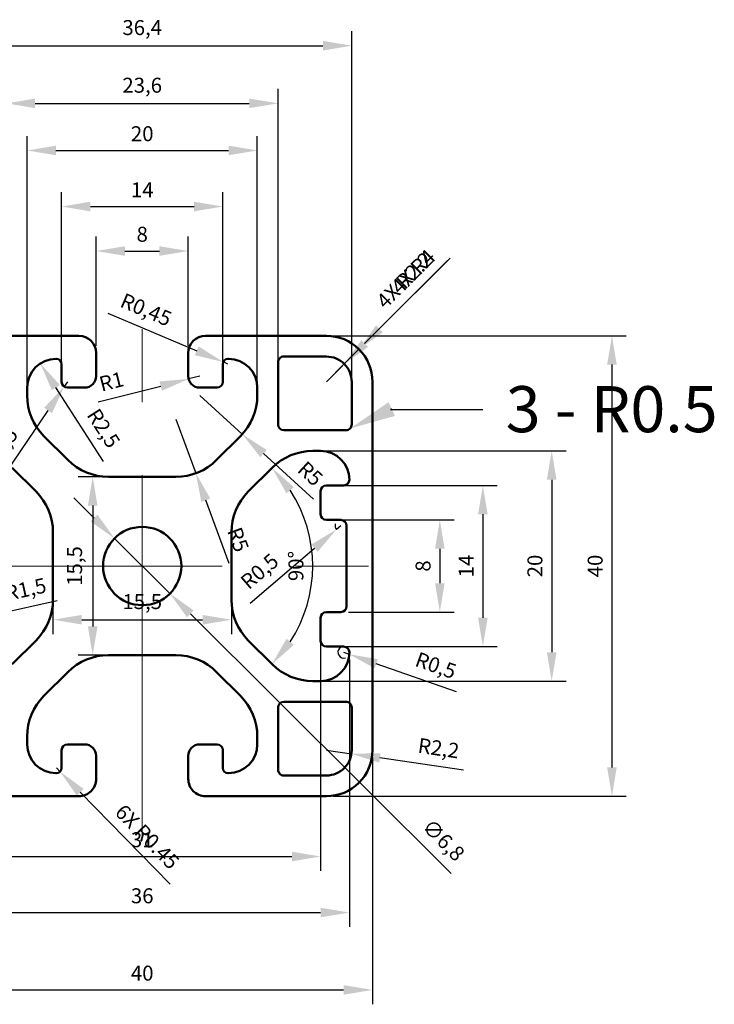
# Model space of a CAD drawing. Units: millimetres. Extents: x 2580.1 to 2672.5, y 2225.2 to 2310.7.
# Tile 2 of 2: x 2612.2 to 2672.5, y 2225.2 to 2310.7. Entities that reach past the tile are written whole.
import ezdxf
from ezdxf import colors
from ezdxf.entities.mleader import LeaderData, LeaderLine
from ezdxf.math import Vec2, Vec3

# ---------------------------------------------------------------- set-up
doc = ezdxf.new("R2010")
doc.units = ezdxf.units.MM
doc.linetypes.add('CENTER', pattern=[50.8, 31.75, -6.35, 6.35, -6.35])
for name, color, linetype, lineweight in [('M-CNTR', 1, 'CENTER', 18), ('M-DIMS', 2, 'Continuous', 25), ('M-OUTL', 7, 'Continuous', 50), ('M-TEXT', 3, 'Continuous', 25)]:
    doc.layers.add(name, color=color, linetype=linetype, lineweight=lineweight)
doc.styles.get("Standard").update_dxf_attribs({"font": 'arial.ttf'})
doc.dimstyles.new('ISO-25', dxfattribs={"dimtxt": 1.3, "dimasz": 2.5, "dimexe": 1.25, "dimexo": 0.625, "dimtad": 1, "dimtxsty": 'Standard', "dimcen": 2.5, "dimadec": 0, "dimazin": 0, "dimtfac": 1, "dimtmove": 0, "dimatfit": 3, "dimfxl": 1, "dimarcsym": 0})

# ---------------------------------------------------------------- blocks, each defined once
blk = doc.blocks.new('*D1')
at = {"layer": 'Defpoints', "color": 0, "transparency": 16777216}
for p in [(2626.849, 2290.611), (2618.849, 2281.743), (2626.849, 2281.743)]:
    blk.add_point(p, dxfattribs=at)
at = {"layer": 'M-DIMS', "color": 0, "lineweight": -2, "transparency": 16777216}
for p, q in [((2618.849, 2282.368), (2618.849, 2291.861)), ((2626.849, 2282.368), (2626.849, 2291.861)), ((2621.349, 2290.611), (2624.349, 2290.611))]:
    blk.add_line(p, q, dxfattribs=at)
at = {"layer": 'M-DIMS', "color": 0, "transparency": 16777216}
for points in [[(2621.349, 2291.028), (2621.349, 2290.194), (2618.849, 2290.611)], [(2624.349, 2291.028), (2624.349, 2290.194), (2626.849, 2290.611)]]:
    blk.add_solid(points, dxfattribs=at)
at = {"layer": 'M-DIMS', "color": 0, "transparency": 16777216, "insert": (2622.849, 2291.9), "char_height": 1.3, "attachment_point": 5}
blk.add_mtext('8', dxfattribs=at)
blk = doc.blocks.new('*D2')
at = {"layer": 'Defpoints', "color": 0, "transparency": 16777216}
for p in [(2629.849, 2294.477), (2615.849, 2280.018), (2629.849, 2280.018)]:
    blk.add_point(p, dxfattribs=at)
at = {"layer": 'M-DIMS', "color": 0, "lineweight": -2, "transparency": 16777216}
for p, q in [((2615.849, 2280.643), (2615.849, 2295.727)), ((2629.849, 2280.643), (2629.849, 2295.727)), ((2618.349, 2294.477), (2627.349, 2294.477))]:
    blk.add_line(p, q, dxfattribs=at)
at = {"layer": 'M-DIMS', "color": 0, "transparency": 16777216}
for points in [[(2618.349, 2294.894), (2618.349, 2294.061), (2615.849, 2294.477)], [(2627.349, 2294.894), (2627.349, 2294.061), (2629.849, 2294.477)]]:
    blk.add_solid(points, dxfattribs=at)
at = {"layer": 'M-DIMS', "color": 0, "transparency": 16777216, "insert": (2622.849, 2295.755), "char_height": 1.3, "attachment_point": 5}
blk.add_mtext('14', dxfattribs=at)
blk = doc.blocks.new('*D3')
at = {"layer": 'Defpoints', "color": 0, "transparency": 16777216}
for p in [(2632.849, 2299.349), (2612.849, 2278.404), (2632.849, 2278.404)]:
    blk.add_point(p, dxfattribs=at)
at = {"layer": 'M-DIMS', "color": 0, "lineweight": -2, "transparency": 16777216}
for p, q in [((2612.849, 2279.029), (2612.849, 2300.599)), ((2632.849, 2279.029), (2632.849, 2300.599)), ((2615.349, 2299.349), (2630.349, 2299.349))]:
    blk.add_line(p, q, dxfattribs=at)
at = {"layer": 'M-DIMS', "color": 0, "transparency": 16777216}
for points in [[(2615.349, 2299.766), (2615.349, 2298.932), (2612.849, 2299.349)], [(2630.349, 2299.766), (2630.349, 2298.932), (2632.849, 2299.349)]]:
    blk.add_solid(points, dxfattribs=at)
at = {"layer": 'M-DIMS', "color": 0, "transparency": 16777216, "insert": (2622.849, 2300.638), "char_height": 1.3, "attachment_point": 5}
blk.add_mtext('20', dxfattribs=at)
blk = doc.blocks.new('*D4')
at = {"layer": 'Defpoints', "color": 0, "transparency": 16777216}
for p in [(2634.649, 2303.442), (2611.049, 2278.243), (2634.649, 2278.243)]:
    blk.add_point(p, dxfattribs=at)
at = {"layer": 'M-DIMS', "color": 0, "lineweight": -2, "transparency": 16777216}
for p, q in [((2611.049, 2278.868), (2611.049, 2304.692)), ((2634.649, 2278.868), (2634.649, 2304.692)), ((2613.549, 2303.442), (2632.149, 2303.442))]:
    blk.add_line(p, q, dxfattribs=at)
at = {"layer": 'M-DIMS', "color": 0, "transparency": 16777216}
for points in [[(2613.549, 2303.859), (2613.549, 2303.026), (2611.049, 2303.442)], [(2632.149, 2303.859), (2632.149, 2303.026), (2634.649, 2303.442)]]:
    blk.add_solid(points, dxfattribs=at)
at = {"layer": 'M-DIMS', "color": 0, "transparency": 16777216, "insert": (2622.849, 2304.849), "char_height": 1.3, "attachment_point": 5}
blk.add_mtext('23,6', dxfattribs=at)
blk = doc.blocks.new('*D5')
at = {"layer": 'Defpoints', "color": 0, "transparency": 16777216}
for p in [(2641.049, 2308.452), (2604.649, 2277.393), (2641.049, 2277.393)]:
    blk.add_point(p, dxfattribs=at)
at = {"layer": 'M-DIMS', "color": 0, "lineweight": -2, "transparency": 16777216}
for p, q in [((2604.649, 2278.018), (2604.649, 2309.702)), ((2641.049, 2278.018), (2641.049, 2309.702)), ((2607.149, 2308.452), (2638.549, 2308.452))]:
    blk.add_line(p, q, dxfattribs=at)
at = {"layer": 'M-DIMS', "color": 0, "transparency": 16777216}
for points in [[(2607.149, 2308.869), (2607.149, 2308.036), (2604.649, 2308.452)], [(2638.549, 2308.869), (2638.549, 2308.036), (2641.049, 2308.452)]]:
    blk.add_solid(points, dxfattribs=at)
at = {"layer": 'M-DIMS', "color": 0, "transparency": 16777216, "insert": (2622.849, 2309.859), "char_height": 1.3, "attachment_point": 5}
blk.add_mtext('36,4', dxfattribs=at)
blk = doc.blocks.new('*D11')
at = {"layer": 'Defpoints', "color": 0, "transparency": 16777216}
for p in [(2602.849, 2247.243), (2642.849, 2247.243), (2642.849, 2226.409)]:
    blk.add_point(p, dxfattribs=at)
at = {"layer": 'M-DIMS', "color": 0, "lineweight": -2, "transparency": 16777216}
for p, q in [((2602.849, 2246.618), (2602.849, 2225.159)), ((2642.849, 2246.618), (2642.849, 2225.159)), ((2605.349, 2226.409), (2640.349, 2226.409))]:
    blk.add_line(p, q, dxfattribs=at)
at = {"layer": 'M-DIMS', "color": 0, "transparency": 16777216}
for points in [[(2605.349, 2226.826), (2605.349, 2225.992), (2602.849, 2226.409)], [(2640.349, 2226.826), (2640.349, 2225.992), (2642.849, 2226.409)]]:
    blk.add_solid(points, dxfattribs=at)
at = {"layer": 'M-DIMS', "color": 0, "transparency": 16777216, "insert": (2622.849, 2227.698), "char_height": 1.3, "attachment_point": 5}
blk.add_mtext('40', dxfattribs=at)
blk = doc.blocks.new('*D12')
at = {"layer": 'Defpoints', "color": 0, "transparency": 16777216}
for p in [(2607.349, 2257.493), (2638.349, 2257.493), (2638.349, 2238.001)]:
    blk.add_point(p, dxfattribs=at)
at = {"layer": 'M-DIMS', "color": 0, "lineweight": -2, "transparency": 16777216}
for p, q in [((2607.349, 2256.868), (2607.349, 2236.751)), ((2638.349, 2256.868), (2638.349, 2236.751)), ((2609.849, 2238.001), (2635.849, 2238.001))]:
    blk.add_line(p, q, dxfattribs=at)
at = {"layer": 'M-DIMS', "color": 0, "transparency": 16777216}
for points in [[(2609.849, 2238.418), (2609.849, 2237.584), (2607.349, 2238.001)], [(2635.849, 2238.418), (2635.849, 2237.584), (2638.349, 2238.001)]]:
    blk.add_solid(points, dxfattribs=at)
at = {"layer": 'M-DIMS', "color": 0, "transparency": 16777216, "insert": (2622.849, 2239.29), "char_height": 1.3, "attachment_point": 5}
blk.add_mtext('31', dxfattribs=at)
blk = doc.blocks.new('*D13')
at = {"layer": 'Defpoints', "color": 0, "transparency": 16777216}
for p in [(2604.85, 2255.804), (2640.849, 2255.743), (2640.849, 2233.131)]:
    blk.add_point(p, dxfattribs=at)
at = {"layer": 'M-DIMS', "color": 0, "lineweight": -2, "transparency": 16777216}
for p, q in [((2604.85, 2255.179), (2604.85, 2231.881)), ((2640.849, 2255.118), (2640.849, 2231.881)), ((2607.35, 2233.131), (2638.349, 2233.131))]:
    blk.add_line(p, q, dxfattribs=at)
at = {"layer": 'M-DIMS', "color": 0, "transparency": 16777216}
for points in [[(2607.35, 2233.547), (2607.35, 2232.714), (2604.85, 2233.131)], [(2638.349, 2233.547), (2638.349, 2232.714), (2640.849, 2233.131)]]:
    blk.add_solid(points, dxfattribs=at)
at = {"layer": 'M-DIMS', "color": 0, "transparency": 16777216, "insert": (2622.85, 2234.42), "char_height": 1.3, "attachment_point": 5}
blk.add_mtext('36', dxfattribs=at)
blk = doc.blocks.new('*D14')
at = {"layer": 'Defpoints', "color": 0, "transparency": 16777216}
for p in [(2639.474, 2267.243), (2640.141, 2259.245), (2648.704, 2259.245)]:
    blk.add_point(p, dxfattribs=at)
at = {"layer": 'M-DIMS', "color": 0, "lineweight": -2, "transparency": 16777216}
for p, q in [((2640.099, 2267.243), (2649.954, 2267.243)), ((2648.704, 2264.743), (2648.704, 2261.745)), ((2640.766, 2259.245), (2649.954, 2259.245))]:
    blk.add_line(p, q, dxfattribs=at)
at = {"layer": 'M-DIMS', "color": 0, "transparency": 16777216}
for points in [[(2648.287, 2264.743), (2649.12, 2264.743), (2648.704, 2267.243)], [(2648.287, 2261.745), (2649.12, 2261.745), (2648.704, 2259.245)]]:
    blk.add_solid(points, dxfattribs=at)
at = {"layer": 'M-DIMS', "color": 0, "transparency": 16777216, "insert": (2647.415, 2263.244), "char_height": 1.3, "attachment_point": 5, "rotation": 90}
blk.add_mtext('8', dxfattribs=at)
blk = doc.blocks.new('*D15')
at = {"layer": 'Defpoints', "color": 0, "transparency": 16777216}
for p in [(2639.599, 2270.243), (2639.599, 2256.243), (2652.44, 2256.243)]:
    blk.add_point(p, dxfattribs=at)
at = {"layer": 'M-DIMS', "color": 0, "lineweight": -2, "transparency": 16777216}
for p, q in [((2640.224, 2270.243), (2653.69, 2270.243)), ((2652.44, 2267.743), (2652.44, 2258.743)), ((2640.224, 2256.243), (2653.69, 2256.243))]:
    blk.add_line(p, q, dxfattribs=at)
at = {"layer": 'M-DIMS', "color": 0, "transparency": 16777216}
for points in [[(2652.024, 2267.743), (2652.857, 2267.743), (2652.44, 2270.243)], [(2652.024, 2258.743), (2652.857, 2258.743), (2652.44, 2256.243)]]:
    blk.add_solid(points, dxfattribs=at)
at = {"layer": 'M-DIMS', "color": 0, "transparency": 16777216, "insert": (2651.163, 2263.243), "char_height": 1.3, "attachment_point": 5, "rotation": 90}
blk.add_mtext('14', dxfattribs=at)
blk = doc.blocks.new('*D16')
at = {"layer": 'Defpoints', "color": 0, "transparency": 16777216}
for p in [(2637.67, 2273.243), (2637.67, 2253.243), (2658.419, 2253.243)]:
    blk.add_point(p, dxfattribs=at)
at = {"layer": 'M-DIMS', "color": 0, "lineweight": -2, "transparency": 16777216}
for p, q in [((2638.295, 2273.243), (2659.669, 2273.243)), ((2658.419, 2270.743), (2658.419, 2255.743)), ((2638.295, 2253.243), (2659.669, 2253.243))]:
    blk.add_line(p, q, dxfattribs=at)
at = {"layer": 'M-DIMS', "color": 0, "transparency": 16777216}
for points in [[(2658.002, 2270.743), (2658.836, 2270.743), (2658.419, 2273.243)], [(2658.002, 2255.743), (2658.836, 2255.743), (2658.419, 2253.243)]]:
    blk.add_solid(points, dxfattribs=at)
at = {"layer": 'M-DIMS', "color": 0, "transparency": 16777216, "insert": (2657.13, 2263.243), "char_height": 1.3, "attachment_point": 5, "rotation": 90}
blk.add_mtext('20', dxfattribs=at)
blk = doc.blocks.new('*D17')
at = {"layer": 'Defpoints', "color": 0, "transparency": 16777216}
for p in [(2638.849, 2283.243), (2638.849, 2243.243), (2663.65, 2243.243)]:
    blk.add_point(p, dxfattribs=at)
at = {"layer": 'M-DIMS', "color": 0, "lineweight": -2, "transparency": 16777216}
for p, q in [((2639.474, 2283.243), (2664.9, 2283.243)), ((2663.65, 2280.743), (2663.65, 2245.743)), ((2639.474, 2243.243), (2664.9, 2243.243))]:
    blk.add_line(p, q, dxfattribs=at)
at = {"layer": 'M-DIMS', "color": 0, "transparency": 16777216}
for points in [[(2663.234, 2280.743), (2664.067, 2280.743), (2663.65, 2283.243)], [(2663.234, 2245.743), (2664.067, 2245.743), (2663.65, 2243.243)]]:
    blk.add_solid(points, dxfattribs=at)
at = {"layer": 'M-DIMS', "color": 0, "transparency": 16777216, "insert": (2662.362, 2263.243), "char_height": 1.3, "attachment_point": 5, "rotation": 90}
blk.add_mtext('40', dxfattribs=at)
blk = doc.blocks.new('*D18')
at = {"layer": 'Defpoints', "color": 0, "transparency": 16777216}
for p in [(2616.349, 2279.243), (2616.069, 2278.829)]:
    blk.add_point(p, dxfattribs=at)
at = {"layer": 'M-DIMS', "color": 0, "lineweight": -2, "transparency": 16777216}
for p, q in [((2616.349, 2279.243), (2616.069, 2278.829)), ((2610.54, 2270.653), (2614.669, 2276.758))]:
    blk.add_line(p, q, dxfattribs=at)
at = {"layer": 'M-DIMS', "color": 0, "transparency": 16777216}
blk.add_solid([(2614.324, 2276.992), (2615.014, 2276.525), (2616.069, 2278.829)], dxfattribs=at)
at = {"layer": 'M-DIMS', "color": 0, "transparency": 16777216, "insert": (2610.739, 2273.458), "char_height": 1.3, "attachment_point": 5, "rotation": 55.93249}
blk.add_mtext('R0,5', dxfattribs=at)
blk = doc.blocks.new('*D19')
at = {"layer": 'Defpoints', "color": 0, "transparency": 16777216}
for p in [(2613.997, 2280.846), (2615.349, 2278.743)]:
    blk.add_point(p, dxfattribs=at)
at = {"layer": 'M-DIMS', "color": 0, "lineweight": -2, "transparency": 16777216}
blk.add_line((2619.489, 2272.311), (2615.349, 2278.743), dxfattribs=at)
at = {"layer": 'M-DIMS', "color": 0, "transparency": 16777216}
blk.add_solid([(2615.7, 2278.969), (2614.999, 2278.518), (2613.997, 2280.846)], dxfattribs=at)
at = {"layer": 'M-DIMS', "color": 0, "transparency": 16777216, "insert": (2619.353, 2275.12), "char_height": 1.3, "attachment_point": 5, "rotation": 302.75966}
blk.add_mtext('R2,5', dxfattribs=at)
blk = doc.blocks.new('*D20')
at = {"layer": 'Defpoints', "color": 0, "transparency": 16777216}
for p in [(2629.885, 2280.969), (2630.299, 2280.793)]:
    blk.add_point(p, dxfattribs=at)
at = {"layer": 'M-DIMS', "color": 0, "lineweight": -2, "transparency": 16777216}
for p, q in [((2619.866, 2285.212), (2627.583, 2281.944)), ((2630.299, 2280.793), (2629.885, 2280.969))]:
    blk.add_line(p, q, dxfattribs=at)
at = {"layer": 'M-DIMS', "color": 0, "transparency": 16777216}
blk.add_solid([(2627.745, 2282.328), (2627.421, 2281.56), (2629.885, 2280.969)], dxfattribs=at)
at = {"layer": 'M-DIMS', "color": 0, "transparency": 16777216, "insert": (2623.122, 2285.36), "char_height": 1.3, "attachment_point": 5, "rotation": 337.04634}
blk.add_mtext('R0,45', dxfattribs=at)
blk = doc.blocks.new('*D21')
at = {"layer": 'Defpoints', "color": 0, "transparency": 16777216}
for p in [(2627.849, 2278.064), (2631.543, 2274.695)]:
    blk.add_point(p, dxfattribs=at)
at = {"layer": 'M-DIMS', "color": 0, "lineweight": -2, "transparency": 16777216}
for p, q in [((2627.849, 2278.064), (2631.543, 2274.695)), ((2637.717, 2269.063), (2633.39, 2273.01))]:
    blk.add_line(p, q, dxfattribs=at)
at = {"layer": 'M-DIMS', "color": 0, "transparency": 16777216}
blk.add_solid([(2633.671, 2273.318), (2633.11, 2272.702), (2631.543, 2274.695)], dxfattribs=at)
at = {"layer": 'M-DIMS', "color": 0, "transparency": 16777216, "insert": (2637.344, 2271.145), "char_height": 1.3, "attachment_point": 5, "rotation": 317.62952}
blk.add_mtext('R5', dxfattribs=at)
blk = doc.blocks.new('*D22')
at = {"layer": 'Defpoints', "color": 0, "transparency": 16777216}
for p in [(2626.88, 2279.496), (2627.849, 2279.743)]:
    blk.add_point(p, dxfattribs=at)
at = {"layer": 'M-DIMS', "color": 0, "lineweight": -2, "transparency": 16777216}
for p, q in [((2627.849, 2279.743), (2626.88, 2279.496)), ((2619.037, 2277.494), (2624.458, 2278.878))]:
    blk.add_line(p, q, dxfattribs=at)
at = {"layer": 'M-DIMS', "color": 0, "transparency": 16777216}
blk.add_solid([(2624.355, 2279.281), (2624.561, 2278.474), (2626.88, 2279.496)], dxfattribs=at)
at = {"layer": 'M-DIMS', "color": 0, "transparency": 16777216, "insert": (2620.22, 2279.115), "char_height": 1.3, "attachment_point": 5, "rotation": 14.31882}
blk.add_mtext('R1', dxfattribs=at)
blk = doc.blocks.new('*D23')
at = {"layer": 'Defpoints', "color": 0, "transparency": 16777216}
for p in [(2625.778, 2275.993), (2627.508, 2271.302)]:
    blk.add_point(p, dxfattribs=at)
at = {"layer": 'M-DIMS', "color": 0, "lineweight": -2, "transparency": 16777216}
for p, q in [((2625.778, 2275.993), (2627.508, 2271.302)), ((2630.399, 2263.462), (2628.373, 2268.957))]:
    blk.add_line(p, q, dxfattribs=at)
at = {"layer": 'M-DIMS', "color": 0, "transparency": 16777216}
blk.add_solid([(2628.764, 2269.101), (2627.982, 2268.812), (2627.508, 2271.302)], dxfattribs=at)
at = {"layer": 'M-DIMS', "color": 0, "transparency": 16777216, "insert": (2631.025, 2265.481), "char_height": 1.3, "attachment_point": 5, "rotation": 290.2413}
blk.add_mtext('R5', dxfattribs=at)
blk = doc.blocks.new('*D24')
at = {"layer": 'Defpoints', "color": 0, "transparency": 16777216}
for p in [(2604.349, 2257.743), (2605.814, 2258.069)]:
    blk.add_point(p, dxfattribs=at)
at = {"layer": 'M-DIMS', "color": 0, "lineweight": -2, "transparency": 16777216}
for p, q in [((2615.449, 2260.209), (2608.254, 2258.611)), ((2604.349, 2257.743), (2605.814, 2258.069))]:
    blk.add_line(p, q, dxfattribs=at)
blk.add_arc((2604.349, 2257.743), 1.5, 324.77892, 66.12676, dxfattribs=at)
at = {"layer": 'M-DIMS', "color": 0, "transparency": 16777216}
blk.add_solid([(2608.164, 2259.018), (2608.345, 2258.204), (2605.814, 2258.069)], dxfattribs=at)
at = {"layer": 'M-DIMS', "color": 0, "transparency": 16777216, "insert": (2612.767, 2261.054), "char_height": 1.3, "attachment_point": 5, "rotation": 12.5254}
blk.add_mtext('R1,5', dxfattribs=at)
blk = doc.blocks.new('*D25')
at = {"layer": 'Defpoints', "color": 0, "transparency": 16777216}
for p in [(2639.719, 2266.419), (2640.099, 2266.743)]:
    blk.add_point(p, dxfattribs=at)
at = {"layer": 'M-DIMS', "color": 0, "lineweight": -2, "transparency": 16777216}
for p, q in [((2640.099, 2266.743), (2639.719, 2266.419)), ((2632.214, 2260.008), (2637.818, 2264.795))]:
    blk.add_line(p, q, dxfattribs=at)
blk.add_arc((2640.099, 2266.743), 0.5, 161.61972, 220.5034, dxfattribs=at)
at = {"layer": 'M-DIMS', "color": 0, "transparency": 16777216}
blk.add_solid([(2637.548, 2265.112), (2638.089, 2264.478), (2639.719, 2266.419)], dxfattribs=at)
at = {"layer": 'M-DIMS', "color": 0, "transparency": 16777216, "insert": (2633.152, 2262.659), "char_height": 1.3, "attachment_point": 5, "rotation": 40.5034}
blk.add_mtext('R0,5', dxfattribs=at)
blk = doc.blocks.new('*D26')
at = {"layer": 'Defpoints', "color": 0, "transparency": 16777216}
for p in [(2640.349, 2255.743), (2640.821, 2255.578)]:
    blk.add_point(p, dxfattribs=at)
at = {"layer": 'M-DIMS', "color": 0, "lineweight": -2, "transparency": 16777216}
for p, q in [((2640.349, 2255.743), (2640.821, 2255.578)), ((2650.137, 2252.315), (2643.181, 2254.751))]:
    blk.add_line(p, q, dxfattribs=at)
blk.add_arc((2640.349, 2255.743), 0.5, 340.69312, 288.38028, dxfattribs=at)
at = {"layer": 'M-DIMS', "color": 0, "transparency": 16777216}
blk.add_solid([(2643.318, 2255.145), (2643.043, 2254.358), (2640.821, 2255.578)], dxfattribs=at)
at = {"layer": 'M-DIMS', "color": 0, "transparency": 16777216, "insert": (2648.303, 2254.447), "char_height": 1.3, "attachment_point": 5, "rotation": 340.69312}
blk.add_mtext('R0,5', dxfattribs=at)
blk = doc.blocks.new('*D27')
at = {"layer": 'Defpoints', "color": 0, "transparency": 16777216}
for p in [(2634.135, 2271.779), (2632.064, 2269.708), (2637.247, 2260.122), (2632.064, 2256.779), (2634.135, 2254.708)]:
    blk.add_point(p, dxfattribs=at)
at = {"layer": 'M-DIMS', "color": 0, "lineweight": -2, "transparency": 16777216}
blk.add_arc((2625.599, 2263.243), 12.059, 326.89962, 33.10038, dxfattribs=at)
at = {"layer": 'M-DIMS', "color": 0, "transparency": 16777216}
for points in [[(2635.378, 2269.566), (2636.025, 2270.091), (2634.126, 2271.77)], [(2636.025, 2256.395), (2635.378, 2256.92), (2634.126, 2254.716)]]:
    blk.add_solid(points, dxfattribs=at)
at = {"layer": 'M-DIMS', "color": 0, "transparency": 16777216, "insert": (2636.37, 2263.243), "char_height": 1.3, "attachment_point": 5, "rotation": 90}
blk.add_mtext('90°', dxfattribs=at)
blk = doc.blocks.new('*D28')
at = {"layer": 'Defpoints', "color": 0, "transparency": 16777216}
for p in [(2622.849, 2270.993), (2618.549, 2255.493), (2622.849, 2255.493)]:
    blk.add_point(p, dxfattribs=at)
at = {"layer": 'M-DIMS', "color": 0, "lineweight": -2, "transparency": 16777216}
for p, q in [((2622.224, 2270.993), (2617.299, 2270.993)), ((2618.549, 2268.493), (2618.549, 2257.993)), ((2622.224, 2255.493), (2617.299, 2255.493))]:
    blk.add_line(p, q, dxfattribs=at)
at = {"layer": 'M-DIMS', "color": 0, "transparency": 16777216}
for points in [[(2618.132, 2268.493), (2618.966, 2268.493), (2618.549, 2270.993)], [(2618.132, 2257.993), (2618.966, 2257.993), (2618.549, 2255.493)]]:
    blk.add_solid(points, dxfattribs=at)
at = {"layer": 'M-DIMS', "color": 0, "transparency": 16777216, "insert": (2617.143, 2263.243), "char_height": 1.3, "attachment_point": 5, "rotation": 90}
blk.add_mtext('15,5', dxfattribs=at)
blk = doc.blocks.new('*D29')
at = {"layer": 'Defpoints', "color": 0, "transparency": 16777216}
for p in [(2615.099, 2263.243), (2630.599, 2263.243), (2630.599, 2258.574)]:
    blk.add_point(p, dxfattribs=at)
at = {"layer": 'M-DIMS', "color": 0, "lineweight": -2, "transparency": 16777216}
for p, q in [((2615.099, 2262.618), (2615.099, 2257.324)), ((2630.599, 2262.618), (2630.599, 2257.324)), ((2617.599, 2258.574), (2628.099, 2258.574))]:
    blk.add_line(p, q, dxfattribs=at)
at = {"layer": 'M-DIMS', "color": 0, "transparency": 16777216}
for points in [[(2617.599, 2258.99), (2617.599, 2258.157), (2615.099, 2258.574)], [(2628.099, 2258.99), (2628.099, 2258.157), (2630.599, 2258.574)]]:
    blk.add_solid(points, dxfattribs=at)
at = {"layer": 'M-DIMS', "color": 0, "transparency": 16777216, "insert": (2622.849, 2259.98), "char_height": 1.3, "attachment_point": 5}
blk.add_mtext('15,5', dxfattribs=at)
blk = doc.blocks.new('*D30')
at = {"layer": 'Defpoints', "color": 0, "transparency": 16777216}
for p in [(2620.44, 2265.642), (2625.259, 2260.845)]:
    blk.add_point(p, dxfattribs=at)
at = {"layer": 'M-DIMS', "color": 0, "lineweight": -2, "transparency": 16777216}
for p, q in [((2618.668, 2267.406), (2616.896, 2269.17)), ((2620.44, 2265.642), (2625.259, 2260.845)), ((2649.687, 2236.526), (2627.031, 2259.081))]:
    blk.add_line(p, q, dxfattribs=at)
at = {"layer": 'M-DIMS', "color": 0, "transparency": 16777216}
for points in [[(2618.962, 2267.701), (2618.374, 2267.111), (2620.44, 2265.642)], [(2627.325, 2259.376), (2626.737, 2258.786), (2625.259, 2260.845)]]:
    blk.add_solid(points, dxfattribs=at)
at = {"layer": 'M-DIMS', "color": 0, "transparency": 16777216, "insert": (2648.91, 2239.314), "char_height": 1.3, "attachment_point": 5, "rotation": 315.12838}
blk.add_mtext('∅6,8', dxfattribs=at)
blk = doc.blocks.new('*D31')
at = {"layer": 'Defpoints', "color": 0, "transparency": 16777216}
for p in [(2638.849, 2247.243), (2641.026, 2246.927)]:
    blk.add_point(p, dxfattribs=at)
at = {"layer": 'M-DIMS', "color": 0, "lineweight": -2, "transparency": 16777216}
for p, q in [((2638.849, 2247.243), (2641.026, 2246.927)), ((2650.771, 2245.509), (2643.5, 2246.567))]:
    blk.add_line(p, q, dxfattribs=at)
at = {"layer": 'M-DIMS', "color": 0, "transparency": 16777216}
blk.add_solid([(2643.56, 2246.979), (2643.44, 2246.154), (2641.026, 2246.927)], dxfattribs=at)
at = {"layer": 'M-DIMS', "color": 0, "transparency": 16777216, "insert": (2648.575, 2247.249), "char_height": 1.3, "attachment_point": 5, "rotation": 351.72079}
blk.add_mtext('R2,2', dxfattribs=at)
blk = doc.blocks.new('*D32')
at = {"layer": 'Defpoints', "color": 0, "transparency": 16777216}
for p in [(2641.678, 2282.072), (2638.849, 2279.243)]:
    blk.add_point(p, dxfattribs=at)
at = {"layer": 'M-DIMS', "color": 0, "lineweight": -2, "transparency": 16777216}
for p, q in [((2649.588, 2289.982), (2643.446, 2283.84)), ((2638.849, 2279.243), (2641.678, 2282.072))]:
    blk.add_line(p, q, dxfattribs=at)
at = {"layer": 'M-DIMS', "color": 0, "transparency": 16777216}
blk.add_solid([(2643.151, 2284.134), (2643.74, 2283.545), (2641.678, 2282.072)], dxfattribs=at)
at = {"layer": 'M-DIMS', "color": 0, "transparency": 16777216, "insert": (2646.499, 2288.697), "char_height": 1.3, "attachment_point": 5, "rotation": 45.00047}
blk.add_mtext('4X R4', dxfattribs=at)
blk = doc.blocks.new('*D33')
at = {"layer": 'Defpoints', "color": 0, "transparency": 16777216}
for p in [(2640.405, 2280.799), (2638.849, 2279.243)]:
    blk.add_point(p, dxfattribs=at)
at = {"layer": 'M-DIMS', "color": 0, "lineweight": -2, "transparency": 16777216}
for p, q in [((2649.38, 2289.775), (2642.173, 2282.567)), ((2638.849, 2279.243), (2640.405, 2280.799))]:
    blk.add_line(p, q, dxfattribs=at)
at = {"layer": 'M-DIMS', "color": 0, "transparency": 16777216}
blk.add_solid([(2641.878, 2282.861), (2642.467, 2282.272), (2640.405, 2280.799)], dxfattribs=at)
at = {"layer": 'M-DIMS', "color": 0, "transparency": 16777216, "insert": (2645.757, 2287.958), "char_height": 1.3, "attachment_point": 5, "rotation": 45.00085}
blk.add_mtext('4X R2.2', dxfattribs=at)
blk = doc.blocks.new('*D34')
at = {"layer": 'Defpoints', "color": 0, "transparency": 16777216}
for p in [(2615.399, 2245.693), (2615.714, 2245.372)]:
    blk.add_point(p, dxfattribs=at)
at = {"layer": 'M-DIMS', "color": 0, "lineweight": -2, "transparency": 16777216}
for p, q in [((2615.399, 2245.693), (2615.714, 2245.372)), ((2625.286, 2235.596), (2617.463, 2243.586))]:
    blk.add_line(p, q, dxfattribs=at)
at = {"layer": 'M-DIMS', "color": 0, "transparency": 16777216}
blk.add_solid([(2617.761, 2243.877), (2617.166, 2243.294), (2615.714, 2245.372)], dxfattribs=at)
at = {"layer": 'M-DIMS', "color": 0, "transparency": 16777216, "insert": (2623.17, 2239.599), "char_height": 1.3, "attachment_point": 5, "rotation": 314.39624}
blk.add_mtext('6X R0.45', dxfattribs=at)

msp = doc.modelspace()

# ---------------------------------------------------------------- linework, layer by layer
at = {"layer": 'M-CNTR'}
for p, q in [((2622.849, 2239.379), (2622.849, 2287.455)), ((2598.059, 2263.243), (2646.996, 2263.243))]:
    msp.add_line(p, q, dxfattribs=at)
at = {"layer": 'M-OUTL'}
for p, q in [((2618.849, 2279.743), (2618.849, 2281.743)), ((2626.849, 2279.743), (2626.849, 2281.743)), ((2615.399, 2281.243), (2615.349, 2281.243)), ((2630.299, 2281.243), (2630.349, 2281.243)), ((2615.849, 2279.243), (2615.849, 2280.793)), ((2629.849, 2279.243), (2629.849, 2280.793)), ((2612.849, 2278.743), (2612.849, 2278.064)), ((2617.849, 2278.743), (2616.349, 2278.743)), ((2627.849, 2278.743), (2629.349, 2278.743)), ((2632.849, 2278.743), (2632.849, 2278.064)), ((2616.385, 2272.458), (2614.314, 2274.529)), ((2629.314, 2272.458), (2631.385, 2274.529)), ((2637.67, 2273.243), (2638.349, 2273.243)), ((2613.635, 2269.708), (2611.564, 2271.779)), ((2632.064, 2269.708), (2634.135, 2271.779)), ((2622.849, 2270.993), (2619.92, 2270.993)), ((2622.849, 2270.993), (2625.778, 2270.993)), ((2640.849, 2270.743), (2640.849, 2270.743)), ((2638.349, 2267.743), (2638.349, 2269.743)), ((2638.849, 2270.243), (2640.349, 2270.243)), ((2638.849, 2267.243), (2640.099, 2267.243)), ((2642.849, 2259.243), (2642.849, 2267.243)), ((2640.599, 2266.743), (2640.599, 2259.743)), ((2615.099, 2266.172), (2615.099, 2260.314)), ((2630.599, 2263.243), (2630.599, 2266.172)), ((2630.599, 2263.243), (2630.599, 2260.314)), ((2638.349, 2258.743), (2638.349, 2256.743)), ((2638.849, 2259.243), (2640.099, 2259.243)), ((2613.635, 2256.779), (2611.564, 2254.708)), ((2632.064, 2256.779), (2634.135, 2254.708)), ((2638.849, 2256.243), (2640.349, 2256.243)), ((2622.849, 2255.493), (2619.92, 2255.493)), ((2622.849, 2255.493), (2625.778, 2255.493)), ((2616.385, 2254.029), (2614.314, 2251.958)), ((2629.314, 2254.029), (2631.385, 2251.958)), ((2637.67, 2253.243), (2638.349, 2253.243)), ((2612.849, 2248.422), (2612.849, 2247.743)), ((2632.849, 2248.422), (2632.849, 2247.743)), ((2617.849, 2247.743), (2616.349, 2247.743)), ((2627.849, 2247.743), (2629.349, 2247.743)), ((2615.849, 2247.243), (2615.849, 2245.693)), ((2629.849, 2247.243), (2629.849, 2245.693)), ((2615.399, 2245.243), (2615.349, 2245.243)), ((2630.299, 2245.243), (2630.349, 2245.243))]:
    msp.add_line(p, q, dxfattribs=at)
for points in [[(2607.349, 2269.743), (2607.349, 2268.243, -0.414214), (2606.349, 2267.243), (2604.349, 2267.243, -0.414214), (2602.849, 2268.743), (2602.849, 2279.243, -0.414214), (2606.849, 2283.243), (2617.349, 2283.243)], [(2628.349, 2283.243), (2638.849, 2283.243, -0.414214), (2642.849, 2279.243), (2642.849, 2267.243)], [(2634.649, 2275.543), (2634.649, 2280.943, -0.414214), (2635.149, 2281.443), (2638.849, 2281.443, -0.414214), (2641.049, 2279.243), (2641.049, 2275.543, -0.414214), (2640.549, 2275.043), (2635.149, 2275.043)], [(2618.849, 2246.743), (2618.849, 2244.743, -0.414214), (2617.349, 2243.243), (2606.849, 2243.243, -0.414214), (2602.849, 2247.243), (2602.849, 2257.743, -0.414214), (2604.349, 2259.243), (2606.349, 2259.243)], [(2642.849, 2259.243), (2642.849, 2247.243, -0.414214), (2638.849, 2243.243), (2628.349, 2243.243, -0.414214), (2626.849, 2244.743), (2626.849, 2246.743)], [(2635.149, 2251.443), (2640.549, 2251.443, -0.414214), (2641.049, 2250.943), (2641.049, 2247.243, -0.414214), (2638.849, 2245.043), (2635.149, 2245.043, -0.414214), (2634.649, 2245.543), (2634.649, 2250.943)]]:
    msp.add_lwpolyline(points, format="xyb", dxfattribs=at)
msp.add_circle((2622.849, 2263.243), 3.4, dxfattribs=at)
for centre, radius, start, end in [((2617.349, 2281.743), 1.5, 0, 90), ((2628.349, 2281.743), 1.5, 90, 180), ((2615.349, 2278.743), 2.5, 90, 180), ((2615.399, 2280.793), 0.45, 0, 90), ((2630.299, 2280.793), 0.45, 90, 180), ((2630.349, 2278.743), 2.5, 0, 90), ((2616.349, 2279.243), 0.5, 180, 270), ((2617.849, 2279.743), 1, 270, 0), ((2627.849, 2279.743), 1, 180, 270), ((2629.349, 2279.243), 0.5, 270, 0), ((2617.849, 2278.064), 5, 180, 225), ((2627.849, 2278.064), 5, 315, 0), ((2635.149, 2275.543), 0.5, 180, 270), ((2637.67, 2268.243), 5, 90, 135), ((2638.349, 2270.743), 2.5, 0, 90), ((2619.92, 2275.993), 5, 225, 270), ((2625.778, 2275.993), 5, 270, 315), ((2640.349, 2270.743), 0.5, 270, 0), ((2638.849, 2269.743), 0.5, 90, 180), ((2610.099, 2266.172), 5, 0, 45), ((2635.599, 2266.172), 5, 135, 180), ((2638.849, 2267.743), 0.5, 180, 270), ((2640.099, 2266.743), 0.5, 0, 90), ((2610.099, 2260.314), 5, 315, 0), ((2635.599, 2260.314), 5, 180, 225), ((2640.099, 2259.743), 0.5, 270, 0), ((2638.849, 2258.743), 0.5, 90, 180), ((2638.849, 2256.743), 0.5, 180, 270), ((2640.349, 2255.743), 0.5, 0, 90), ((2619.92, 2250.493), 5, 90, 135), ((2625.778, 2250.493), 5, 45, 90), ((2638.349, 2255.743), 2.5, 270, 0), ((2637.67, 2258.243), 5, 225, 270), ((2617.849, 2248.422), 5, 135, 180), ((2627.849, 2248.422), 5, 0, 45), ((2635.149, 2250.943), 0.5, 90, 180), ((2615.349, 2247.743), 2.5, 180, 270), ((2616.349, 2247.243), 0.5, 90, 180), ((2617.849, 2246.743), 1, 360, 90), ((2627.849, 2246.743), 1, 90, 180), ((2629.349, 2247.243), 0.5, 0, 90), ((2630.349, 2247.743), 2.5, 270, 0), ((2615.399, 2245.693), 0.45, 270, 0), ((2630.299, 2245.693), 0.45, 180, 270)]:
    msp.add_arc(centre, radius, start, end, dxfattribs=at)

# ---------------------------------------------------------------- dimensions: what is measured, and where the dimension line sits
at = {"layer": 'M-DIMS'}
for base, p1, p2, picture, middle in [((2641.049, 2308.452), (2604.649, 2277.393), (2641.049, 2277.393), '*D5', (2622.849, 2309.859)), ((2634.649, 2303.442), (2611.049, 2278.243), (2634.649, 2278.243), '*D4', (2622.849, 2304.849)), ((2632.849, 2299.349), (2612.849, 2278.404), (2632.849, 2278.404), '*D3', (2622.849, 2300.638)), ((2629.849, 2294.477), (2615.849, 2280.018), (2629.849, 2280.018), '*D2', (2622.849, 2295.755)), ((2626.849, 2290.611), (2618.849, 2281.743), (2626.849, 2281.743), '*D1', (2622.849, 2291.9)), ((2630.599, 2258.574), (2615.099, 2263.243), (2630.599, 2263.243), '*D29', (2622.849, 2259.98)), ((2638.349, 2238.001), (2607.349, 2257.493), (2638.349, 2257.493), '*D12', (2622.849, 2239.29)), ((2640.849, 2233.131), (2604.85, 2255.804), (2640.849, 2255.743), '*D13', (2622.85, 2234.42)), ((2642.849, 2226.409), (2602.849, 2247.243), (2642.849, 2247.243), '*D11', (2622.849, 2227.698))]:
    dim = msp.add_linear_dim(base=base, p1=p1, p2=p2, dimstyle='ISO-25', override={"dimclrd": 0, "dimclre": 0, "dimclrt": 0}, dxfattribs=at)
    dim.commit()
    dim.dimension.update_dxf_attribs({"geometry": picture, "text_midpoint": middle})
for center, mpoint, text, override, picture, middle in [((2638.849, 2279.243), (2641.678, 2282.072), '4X <>', {"dimdec": 0, "dimlfac": 1, "dimrnd": 0, "dimzin": 0, "dimdsep": 46, "dimlunit": 2}, '*D32', (2646.499, 2288.697)), ((2638.849, 2279.243), (2640.405, 2280.799), '4X <>', {"dimdec": 1, "dimlfac": 1, "dimrnd": 0, "dimzin": 0, "dimdsep": 46, "dimlunit": 2}, '*D33', (2645.757, 2287.958)), ((2615.399, 2245.693), (2615.714, 2245.372), '6X <>', {"dimdec": 2, "dimlfac": 1, "dimrnd": 0, "dimzin": 0, "dimdsep": 46, "dimlunit": 2}, '*D34', (2623.17, 2239.599))]:
    dim = msp.add_radius_dim(center=center, mpoint=mpoint, text=text, dimstyle='ISO-25', override=override, dxfattribs=at)
    dim.commit()
    dim.dimension.update_dxf_attribs({"geometry": picture, "text_midpoint": middle})
for center, mpoint, picture, middle in [((2630.299, 2280.793), (2629.885, 2280.969), '*D20', (2623.122, 2285.36)), ((2627.849, 2279.743), (2626.88, 2279.496), '*D22', (2620.22, 2279.115)), ((2616.349, 2279.243), (2616.069, 2278.829), '*D18', (2610.739, 2273.458)), ((2627.849, 2278.064), (2631.543, 2274.695), '*D21', (2637.344, 2271.145)), ((2625.778, 2275.993), (2627.508, 2271.302), '*D23', (2631.025, 2265.481)), ((2640.099, 2266.743), (2639.719, 2266.419), '*D25', (2633.152, 2262.659)), ((2604.349, 2257.743), (2605.814, 2258.069), '*D24', (2612.767, 2261.054)), ((2640.349, 2255.743), (2640.821, 2255.578), '*D26', (2648.303, 2254.447)), ((2638.849, 2247.243), (2641.026, 2246.927), '*D31', (2648.575, 2247.249))]:
    dim = msp.add_radius_dim(center=center, mpoint=mpoint, dimstyle='ISO-25', override={"dimclrd": 0, "dimclre": 0, "dimclrt": 0}, dxfattribs=at)
    dim.commit()
    dim.dimension.update_dxf_attribs({"geometry": picture, "text_midpoint": middle})
for base, p1, p2, picture, middle in [((2663.65, 2243.243), (2638.849, 2283.243), (2638.849, 2243.243), '*D17', (2662.362, 2263.243)), ((2658.419, 2253.243), (2637.67, 2273.243), (2637.67, 2253.243), '*D16', (2657.13, 2263.243)), ((2618.549, 2255.493), (2622.849, 2270.993), (2622.849, 2255.493), '*D28', (2617.143, 2263.243)), ((2652.44, 2256.243), (2639.599, 2270.243), (2639.599, 2256.243), '*D15', (2651.163, 2263.243)), ((2648.704, 2259.245), (2639.474, 2267.243), (2640.141, 2259.245), '*D14', (2647.415, 2263.244))]:
    dim = msp.add_linear_dim(base=base, p1=p1, p2=p2, angle=90, dimstyle='ISO-25', override={"dimclrd": 0, "dimclre": 0, "dimclrt": 0}, dxfattribs=at)
    dim.commit()
    dim.dimension.update_dxf_attribs({"geometry": picture, "text_midpoint": middle})
dim = msp.add_radius_dim(center=(2615.349, 2278.743), mpoint=(2613.997, 2280.846), dimstyle='ISO-25', override={"dimclrd": 0, "dimclre": 0, "dimclrt": 0}, dxfattribs=at)
dim.commit()
dim.dimension.update_dxf_attribs({"geometry": '*D19', "text_midpoint": (2618.171, 2274.359), "dimtype": 164})
dim = msp.add_angular_dim_2l(base=(2637.247, 2260.122), line1=((2632.064, 2256.779), (2634.135, 2254.708)), line2=((2632.064, 2269.708), (2634.135, 2271.779)), dimstyle='ISO-25', override={"dimclrd": 0, "dimclre": 0, "dimclrt": 0}, dxfattribs=at)
dim.commit()
dim.dimension.update_dxf_attribs({"geometry": '*D27', "text_midpoint": (2636.37, 2263.243)})
dim = msp.add_diameter_dim_2p(p1=(2620.44, 2265.642), p2=(2625.259, 2260.845), dimstyle='ISO-25', override={"dimclrd": 0, "dimclre": 0, "dimclrt": 0}, dxfattribs=at)
dim.commit()
dim.dimension.update_dxf_attribs({"geometry": '*D30', "text_midpoint": (2647.903, 2238.302), "dimtype": 163})

# ---------------------------------------------------------------- leaders
at = {"layer": 'M-TEXT'}
ml = msp.add_multileader_mtext('Standard', dxfattribs=at)
ml.set_content('3 - R0.5', color=256)
ml.set_leader_properties()
ml.build(insert=Vec2(0, 0))
ctx = ml.context
ctx.base_point, ctx.plane_origin = Vec3(2652.428, 2276.834), Vec3(2640.903, 2275.19)
notes = []
notes.append((ctx, [(0, (1, 1, 0), (2644.428, 2276.834), (1, 0), 8, [(0, [(2640.903, 2275.19)], 0, [])])]))
ctx.mtext.insert, ctx.mtext.flow_direction = Vec3(2654.428, 2278.87), 5
for ctx, leaders in notes:
    for number, flags, end, landing, length, lines in leaders:
        leader = LeaderData()
        leader.index, (leader.has_last_leader_line, leader.has_dogleg_vector, leader.attachment_direction) = number, flags
        leader.last_leader_point, leader.dogleg_vector, leader.dogleg_length = Vec3(end), Vec3(landing), length
        for number, points, colour, breaks in lines:
            line = LeaderLine()
            line.index, line.vertices, line.color, line.breaks = number, Vec3.list(points), colors.encode_raw_color(colour), breaks
            leader.lines.append(line)
        ctx.leaders.append(leader)

doc.saveas('drawing.dxf')
